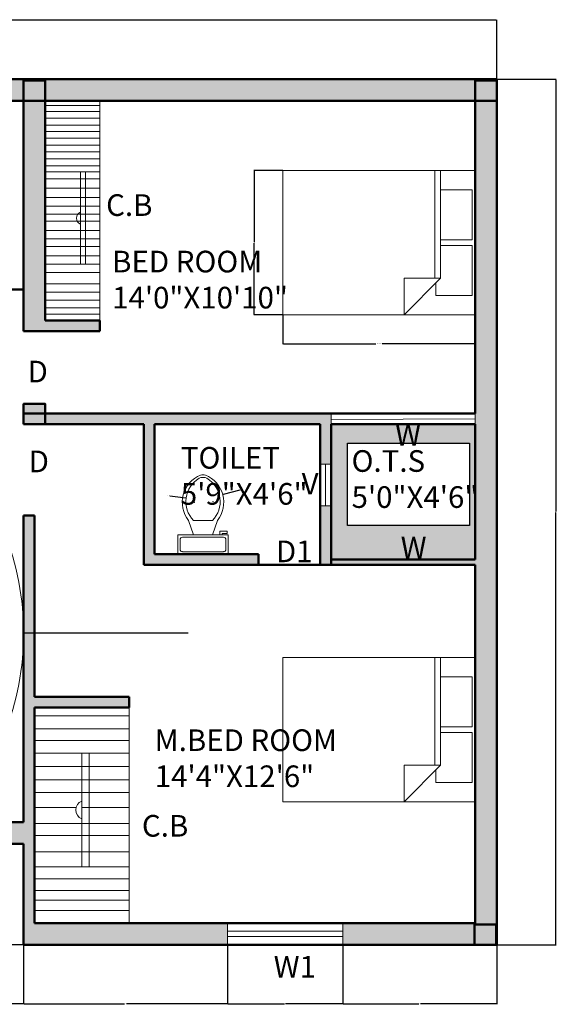
# Model space of a CAD drawing. Units: inches. Extents: x 1099 to 1629, y 1139 to 1548.
# Tile 3 of 3: x 1405 to 1629, y 1139 to 1548. Entities that reach past the tile are written whole.
import ezdxf

# ---------------------------------------------------------------- set-up
doc = ezdxf.new("R2010")
doc.units = ezdxf.units.IN
for name, color, linetype, lineweight in [('A-ANNO-DIMS', 2, 'Continuous', 18), ('A-ANNO-TEXT', 7, 'Continuous', 18), ('A-AREA-IDEN', 7, 'Continuous', 18), ('A-FLOR', 7, 'Continuous', 25), ('A-FLOR-FIXT', 9, 'Continuous', 20), ('A-FLOR-PATT', 3, 'Continuous', 13), ('A-FURN', 8, 'Continuous', 20), ('A-FURN-FIXD', 2, 'Continuous', 18), ('A-WALL', 1, 'Continuous', 50)]:
    doc.layers.add(name, color=color, linetype=linetype, lineweight=lineweight)
for name, color, linetype, lineweight, true_color in [('A-COLS', 177, 'Continuous', 50, 0x293189), ('A-GLAZ', 177, 'Continuous', 20, 0x293189), ('A-WALL-PATT', 244, 'Continuous', 13, 0x991b1e)]:
    doc.layers.add(name, color=color, linetype=linetype, lineweight=lineweight, true_color=true_color)
doc.styles.get("Standard").update_dxf_attribs({"font": 'arial.ttf'})
doc.dimstyles.get("Standard").update_dxf_attribs({"dimtxt": 0.18, "dimasz": 0.18, "dimexe": 0.18, "dimexo": 0.0625, "dimgap": 0.09, "dimtad": 0, "dimtih": 1, "dimtoh": 1, "dimdec": 4, "dimzin": 0, "dimdsep": 46, "dimtxsty": 'Standard', "dimcen": 0.09, "dimadec": 0, "dimazin": 0, "dimtfac": 1, "dimtdec": 4, "dimtofl": 0, "dimtmove": 0, "dimatfit": 3, "dimfxl": 1, "dimtolj": 1, "dimtzin": 0, "dimarcsym": 0})

# ---------------------------------------------------------------- blocks, each defined once
blk = doc.blocks.new('Bed - Queen')
for p, q in [((0, -80.00003), (0, 0)), ((0, 0), (59.99999, 0)), ((59.99999, 0), (59.99999, -80.00003)), ((7.99999, -1.2), (28.79998, -1.2)), ((7.99999, -14.4), (7.99999, -1.2)), ((28.79998, -1.2), (28.79998, -14.4)), ((31.19999, -1.2), (51.99999, -1.2)), ((31.19999, -14.4), (31.19999, -1.2)), ((51.99999, -1.2), (51.99999, -16.4)), ((0, -14.4), (44.8, -14.4)), ((59.99999, -29.6), (44.8, -14.4)), ((44.8, -14.4), (44.8, -29.6)), ((44.8, -16.8), (0, -16.8)), ((51.99999, -16.4), (46.79936, -16.4)), ((44.8, -29.6), (59.99999, -29.6)), ((59.99999, -80.00003), (0, -80.00003))]:
    blk.add_line(p, q)
blk = doc.blocks.new('Toilet - top')
for p, q in [((9.5, -6), (9.5, -2)), ((-8, -8.5), (-8, -8)), ((-7, -8), (-7, -9.5)), ((-4, -8), (-6, -14)), ((4, -8), (6, -14)), ((-10, -8.5), (-8, -8.5)), ((-10, -9.5), (-10, -8.5)), ((-7, -9.5), (-10, -9.5)), ((4, -14), (-4, -14))]:
    blk.add_line(p, q)
blk.add_lwpolyline([(10.5, -8), (10.5, 0), (-10.5, 0), (-10.5, -8)], close=True)
for points in [[(-9.5, -2), (-9.5, -6)], [(8.5, -1), (-8.5, -1)], [(-8.5, -7), (8.5, -7)]]:
    blk.add_lwpolyline(points)
for centre, radius, start, end in [((-8.62, -1.88), 0.884, 81.8699, 188.1301), ((8.62, -1.88), 0.884, 351.8699, 98.1301), ((-8.62, -6.12), 0.884, 171.8699, 278.1301), ((8.62, -6.12), 0.884, 261.8699, 8.1301), ((3.52, -21.58), 12.17, 141.4691, 247.9714), ((4.2, -21.82), 11.33, 136.3677, 238.9468), ((-3.52, -21.58), 12.17, 292.0284, 38.5307), ((-4.2, -21.82), 11.33, 301.053, 43.6321), ((0, -27.88), 4, 245.7318, 294.2682), ((0, -29), 4, 254.8605, 285.1395)]:
    blk.add_arc(centre, radius, start, end)
blk = doc.blocks.new('Sofa - Roundback 7 ft.')
for p, q in [((-12.00002, -32.4421), (-12.00003, -6.5971)), ((11.99997, -32.4421), (11.99998, -6.5971)), ((-36.000027, -34), (-36.000027, -11.4696)), ((35.99998, -34), (35.99998, -11.4696)), ((-35.999844, -13.3819), (35.9998, -13.3819)), ((-36.000027, -32.4421), (35.99998, -32.4421))]:
    blk.add_line(p, q)
for points in [[(-36.000027, -34), (-42.000027, -34), (-42.000027, -8)], [(41.99998, -8), (41.99998, -34), (35.99998, -34)]]:
    blk.add_lwpolyline(points)
for centre, radius, start, end in [((0, -114.25), 114.25, 68.43141, 111.5686), ((-0.00001, -127.1968), 121.1968, 72.72033, 107.2797)]:
    blk.add_arc(centre, radius, start, end)
blk = doc.blocks.new('COL-RECT-9IN')
h = blk.add_hatch(color=256)
h.dxf.hatch_style = 1
h.paths.add_polyline_path([(9, 8.44), (0, 8.44), (0, 0), (9, 0)])
blk.add_lwpolyline([(0, 0), (9, 0), (9, 8.44), (0, 8.44)], close=True)
blk = doc.blocks.new('*D9')
at = {"layer": 'A-ANNO-DIMS', "color": 0, "lineweight": -2, "transparency": 16777216}
for p, q in [((1515.1, 1425.57), (1515.1, 1413.45)), ((1595.1, 1425.57), (1595.1, 1413.45)), ((1515.28, 1413.63), (1553.8, 1413.63)), ((1594.92, 1413.63), (1556.4, 1413.63))]:
    blk.add_line(p, q, dxfattribs=at)
at = {"layer": 'A-ANNO-DIMS', "color": 0, "lineweight": 100, "transparency": 16777216}
for points in [[(1515.28, 1413.66), (1515.28, 1413.6), (1515.1, 1413.63)], [(1594.92, 1413.66), (1594.92, 1413.6), (1595.1, 1413.63)]]:
    blk.add_solid(points, dxfattribs=at)
at = {"layer": 'Defpoints', "color": 0, "lineweight": 100, "transparency": 16777216}
for p in [(1515.1, 1425.63), (1595.1, 1425.63), (1595.1, 1413.63)]:
    blk.add_point(p, dxfattribs=at)
at = {"layer": 'A-ANNO-DIMS', "color": 0, "transparency": 16777216, "insert": (1555.1, 1413.63), "char_height": 0.18, "attachment_point": 5}
blk.add_mtext('\\A1;QUEEN BED 80 TYP.', dxfattribs=at)
blk = doc.blocks.new('*D10')
at = {"layer": 'A-ANNO-DIMS', "color": 0, "lineweight": -2, "transparency": 16777216}
for p, q in [((1515.04, 1485.63), (1502.92, 1485.63)), ((1503.1, 1485.45), (1503.1, 1455.81)), ((1503.1, 1425.81), (1503.1, 1455.45)), ((1515.04, 1425.63), (1502.92, 1425.63))]:
    blk.add_line(p, q, dxfattribs=at)
at = {"layer": 'A-ANNO-DIMS', "color": 0, "lineweight": 100, "transparency": 16777216}
for points in [[(1503.07, 1485.45), (1503.13, 1485.45), (1503.1, 1485.63)], [(1503.07, 1425.81), (1503.13, 1425.81), (1503.1, 1425.63)]]:
    blk.add_solid(points, dxfattribs=at)
at = {"layer": 'Defpoints', "color": 0, "lineweight": 100, "transparency": 16777216}
for p in [(1515.1, 1485.63), (1503.1, 1425.63), (1515.1, 1425.63)]:
    blk.add_point(p, dxfattribs=at)
at = {"layer": 'A-ANNO-DIMS', "color": 0, "transparency": 16777216, "insert": (1503.1, 1455.63), "char_height": 0.18, "attachment_point": 5}
blk.add_mtext('\\A1;60 TYP.', dxfattribs=at)
blk = doc.blocks.new('*D25')
at = {"layer": 'A-ANNO-DIMS', "color": 0, "lineweight": -2, "transparency": 16777216}
for p, q in [((1124.1, 1523.69), (1124.1, 1548.41)), ((1124.28, 1548.23), (1363.81, 1548.23)), ((1603.92, 1548.23), (1364.39, 1548.23)), ((1604.1, 1523.69), (1604.1, 1548.41))]:
    blk.add_line(p, q, dxfattribs=at)
at = {"layer": 'A-ANNO-DIMS', "color": 0, "lineweight": 100, "transparency": 16777216}
for points in [[(1124.28, 1548.26), (1124.28, 1548.2), (1124.1, 1548.23)], [(1603.92, 1548.26), (1603.92, 1548.2), (1604.1, 1548.23)]]:
    blk.add_solid(points, dxfattribs=at)
at = {"layer": 'Defpoints', "color": 0, "lineweight": 100, "transparency": 16777216}
for p in [(1604.1, 1548.23), (1124.1, 1523.63), (1604.1, 1523.63)]:
    blk.add_point(p, dxfattribs=at)
at = {"layer": 'A-ANNO-DIMS', "color": 0, "transparency": 16777216, "insert": (1364.1, 1548.23), "char_height": 0.18, "attachment_point": 5}
blk.add_mtext('\\A1;480', dxfattribs=at)
blk = doc.blocks.new('*D26')
at = {"layer": 'A-ANNO-DIMS', "color": 0, "lineweight": -2, "transparency": 16777216}
for p, q in [((1604.16, 1523.63), (1628.88, 1523.63)), ((1628.7, 1523.45), (1628.7, 1343.81)), ((1628.7, 1163.81), (1628.7, 1343.45)), ((1604.16, 1163.63), (1628.88, 1163.63))]:
    blk.add_line(p, q, dxfattribs=at)
at = {"layer": 'A-ANNO-DIMS', "color": 0, "lineweight": 100, "transparency": 16777216}
for points in [[(1628.67, 1523.45), (1628.73, 1523.45), (1628.7, 1523.63)], [(1628.67, 1163.81), (1628.73, 1163.81), (1628.7, 1163.63)]]:
    blk.add_solid(points, dxfattribs=at)
at = {"layer": 'Defpoints', "color": 0, "lineweight": 100, "transparency": 16777216}
for p in [(1604.1, 1523.63), (1628.7, 1523.63), (1604.1, 1163.63)]:
    blk.add_point(p, dxfattribs=at)
at = {"layer": 'A-ANNO-DIMS', "color": 0, "transparency": 16777216, "insert": (1628.7, 1343.63), "char_height": 0.18, "attachment_point": 5}
blk.add_mtext('\\A1;360', dxfattribs=at)
blk = doc.blocks.new('*D30')
at = {"layer": 'A-ANNO-DIMS', "color": 0, "lineweight": -2, "transparency": 16777216}
for p, q in [((1386.73, 1205.57), (1386.73, 1138.85)), ((1407.1, 1163.57), (1407.1, 1138.85)), ((1386.91, 1139.03), (1396.52, 1139.03)), ((1406.92, 1139.03), (1397.31, 1139.03))]:
    blk.add_line(p, q, dxfattribs=at)
at = {"layer": 'A-ANNO-DIMS', "color": 0, "lineweight": 100, "transparency": 16777216}
for points in [[(1386.91, 1139.06), (1386.91, 1139), (1386.73, 1139.03)], [(1406.92, 1139.06), (1406.92, 1139), (1407.1, 1139.03)]]:
    blk.add_solid(points, dxfattribs=at)
at = {"layer": 'Defpoints', "color": 0, "lineweight": 100, "transparency": 16777216}
for p in [(1386.73, 1205.63), (1407.1, 1163.63), (1407.1, 1139.03)]:
    blk.add_point(p, dxfattribs=at)
at = {"layer": 'A-ANNO-DIMS', "color": 0, "transparency": 16777216, "insert": (1396.91, 1139.03), "char_height": 0.18, "attachment_point": 5}
blk.add_mtext('\\A1;20.37', dxfattribs=at)
blk = doc.blocks.new('*D31')
at = {"layer": 'A-ANNO-DIMS', "color": 0, "lineweight": -2, "transparency": 16777216}
for p, q in [((1407.1, 1163.57), (1407.1, 1138.85)), ((1491.99, 1163.57), (1491.99, 1138.85)), ((1407.28, 1139.03), (1449.15, 1139.03)), ((1491.81, 1139.03), (1449.94, 1139.03))]:
    blk.add_line(p, q, dxfattribs=at)
at = {"layer": 'A-ANNO-DIMS', "color": 0, "lineweight": 100, "transparency": 16777216}
for points in [[(1407.28, 1139.06), (1407.28, 1139), (1407.1, 1139.03)], [(1491.81, 1139.06), (1491.81, 1139), (1491.99, 1139.03)]]:
    blk.add_solid(points, dxfattribs=at)
at = {"layer": 'Defpoints', "color": 0, "lineweight": 100, "transparency": 16777216}
for p in [(1407.1, 1163.63), (1491.99, 1163.63), (1491.99, 1139.03)]:
    blk.add_point(p, dxfattribs=at)
at = {"layer": 'A-ANNO-DIMS', "color": 0, "transparency": 16777216, "insert": (1449.54, 1139.03), "char_height": 0.18, "attachment_point": 5}
blk.add_mtext('\\A1;84.89', dxfattribs=at)
blk = doc.blocks.new('*D32')
at = {"layer": 'A-ANNO-DIMS', "color": 0, "lineweight": -2, "transparency": 16777216}
for p, q in [((1491.99, 1163.57), (1491.99, 1138.85)), ((1539.99, 1163.57), (1539.99, 1138.85)), ((1492.17, 1139.03), (1515.77, 1139.03)), ((1539.81, 1139.03), (1516.21, 1139.03))]:
    blk.add_line(p, q, dxfattribs=at)
at = {"layer": 'A-ANNO-DIMS', "color": 0, "lineweight": 100, "transparency": 16777216}
for points in [[(1492.17, 1139.06), (1492.17, 1139), (1491.99, 1139.03)], [(1539.81, 1139.06), (1539.81, 1139), (1539.99, 1139.03)]]:
    blk.add_solid(points, dxfattribs=at)
at = {"layer": 'Defpoints', "color": 0, "lineweight": 100, "transparency": 16777216}
for p in [(1491.99, 1163.63), (1539.99, 1163.63), (1539.99, 1139.03)]:
    blk.add_point(p, dxfattribs=at)
at = {"layer": 'A-ANNO-DIMS', "color": 0, "transparency": 16777216, "insert": (1515.99, 1139.03), "char_height": 0.18, "attachment_point": 5}
blk.add_mtext('\\A1;48', dxfattribs=at)
blk = doc.blocks.new('*D33')
at = {"layer": 'A-ANNO-DIMS', "color": 0, "lineweight": -2, "transparency": 16777216}
for p, q in [((1539.99, 1163.57), (1539.99, 1138.85)), ((1604.1, 1163.57), (1604.1, 1138.85)), ((1540.17, 1139.03), (1571.67, 1139.03)), ((1603.92, 1139.03), (1572.42, 1139.03))]:
    blk.add_line(p, q, dxfattribs=at)
at = {"layer": 'A-ANNO-DIMS', "color": 0, "lineweight": 100, "transparency": 16777216}
for points in [[(1540.17, 1139.06), (1540.17, 1139), (1539.99, 1139.03)], [(1603.92, 1139.06), (1603.92, 1139), (1604.1, 1139.03)]]:
    blk.add_solid(points, dxfattribs=at)
at = {"layer": 'Defpoints', "color": 0, "lineweight": 100, "transparency": 16777216}
for p in [(1539.99, 1163.63), (1604.1, 1163.63), (1604.1, 1139.03)]:
    blk.add_point(p, dxfattribs=at)
at = {"layer": 'A-ANNO-DIMS', "color": 0, "transparency": 16777216, "insert": (1572.04, 1139.03), "char_height": 0.18, "attachment_point": 5}
blk.add_mtext('\\A1;64.11', dxfattribs=at)
blk = doc.blocks.new('*D38')
at = {"layer": 'A-ANNO-DIMS', "color": 0, "lineweight": -2, "transparency": 16777216}
for p, q in [((1292.76, 1293.22), (1292.94, 1293.22)), ((1292.85, 1293.13), (1292.85, 1293.31)), ((1475.65, 1293.22), (1407.28, 1293.22))]:
    blk.add_line(p, q, dxfattribs=at)
at = {"layer": 'A-ANNO-DIMS', "color": 0, "lineweight": 100, "transparency": 16777216}
blk.add_solid([(1407.28, 1293.25), (1407.28, 1293.19), (1407.1, 1293.22)], dxfattribs=at)
at = {"layer": 'Defpoints', "color": 0, "lineweight": 100, "transparency": 16777216}
for p in [(1292.85, 1293.22), (1407.1, 1293.22)]:
    blk.add_point(p, dxfattribs=at)
at = {"layer": 'A-ANNO-DIMS', "color": 0, "transparency": 16777216, "insert": (1476.39, 1293.22), "char_height": 0.18, "attachment_point": 5}
blk.add_mtext('\\A1;2X R114.25', dxfattribs=at)
blk = doc.blocks.new('*D40')
at = {"layer": 'A-ANNO-DIMS', "color": 0, "lineweight": -2, "transparency": 16777216}
for p, q in [((1497.11, 1352.66), (1490.22, 1350.85)), ((1478.19, 1347.71), (1478.37, 1347.71)), ((1478.28, 1347.62), (1478.28, 1347.8))]:
    blk.add_line(p, q, dxfattribs=at)
at = {"layer": 'A-ANNO-DIMS', "color": 0, "lineweight": 100, "transparency": 16777216}
blk.add_solid([(1490.21, 1350.88), (1490.23, 1350.82), (1490.05, 1350.8)], dxfattribs=at)
at = {"layer": 'Defpoints', "color": 0, "lineweight": 100, "transparency": 16777216}
for p in [(1478.28, 1347.71), (1490.05, 1350.8)]:
    blk.add_point(p, dxfattribs=at)
at = {"layer": 'A-ANNO-DIMS', "color": 0, "transparency": 16777216, "insert": (1497.78, 1352.66), "char_height": 0.18, "attachment_point": 5}
blk.add_mtext('\\A1;4X R12.17', dxfattribs=at)
blk = doc.blocks.new('*D41')
at = {"layer": 'A-ANNO-DIMS', "color": 0, "lineweight": -2, "transparency": 16777216}
for p, q in [((1468.03, 1350.36), (1474.59, 1349.48)), ((1485.9, 1347.95), (1486.08, 1347.95)), ((1485.99, 1347.86), (1485.99, 1348.04))]:
    blk.add_line(p, q, dxfattribs=at)
at = {"layer": 'A-ANNO-DIMS', "color": 0, "lineweight": 100, "transparency": 16777216}
blk.add_solid([(1474.59, 1349.51), (1474.58, 1349.45), (1474.77, 1349.46)], dxfattribs=at)
at = {"layer": 'Defpoints', "color": 0, "lineweight": 100, "transparency": 16777216}
for p in [(1474.77, 1349.46), (1485.99, 1347.95)]:
    blk.add_point(p, dxfattribs=at)
at = {"layer": 'A-ANNO-DIMS', "color": 0, "transparency": 16777216, "insert": (1467.35, 1350.36), "char_height": 0.18, "attachment_point": 5}
blk.add_mtext('\\A1;4X R11.33', dxfattribs=at)

msp = doc.modelspace()

# ---------------------------------------------------------------- hatches: boundary and pattern name
at = {"layer": 'A-FLOR-PATT'}
h = msp.add_hatch(color=256, dxfattribs=at)
h.dxf.hatch_style = 1
h.paths.add_polyline_path([(1595.099, 1380.128), (1535.099, 1380.128), (1535.099, 1326.128), (1535.099, 1323.878), (1595.099, 1323.878)])
h.paths.add_polyline_path([(1542.026, 1338.035), (1542.026, 1372.311), (1592.789, 1372.311), (1592.789, 1338.035)], flags=16)
h.paths.add_polyline_path([(1540.803, 1340.228), (1595.472, 1340.228), (1595.472, 1373.811), (1540.803, 1373.811)], flags=9)
at = {"layer": 'A-WALL-PATT'}
h = msp.add_hatch(color=256, dxfattribs=at)
h.dxf.hatch_style = 1
h.paths.add_polyline_path([(1407.099, 1523.072), (1416.099, 1523.072), (1416.099, 1514.628), (1595.099, 1514.628), (1595.099, 1523.072), (1604.099, 1523.072), (1604.099, 1523.628), (1124.099, 1523.628), (1124.099, 1172.072), (1133.099, 1172.072), (1133.099, 1361.628), (1265.099, 1361.628), (1265.099, 1301.628), (1269.599, 1301.628), (1269.599, 1366.128), (1133.099, 1366.128), (1133.099, 1462.128), (1169.127, 1462.128), (1169.127, 1466.628), (1133.099, 1466.628), (1133.099, 1514.628), (1265.099, 1514.628), (1265.099, 1514.872), (1265.099, 1523.316), (1274.099, 1523.316), (1274.099, 1514.628), (1326.599, 1514.628), (1326.599, 1508.465), (1331.099, 1508.465), (1331.099, 1514.628), (1407.099, 1514.628)])
h.paths.add_polyline_path([(1604.099, 1514.628), (1595.099, 1514.628), (1595.099, 1384.628), (1595.099, 1380.128), (1595.099, 1323.878), (1535.099, 1323.878), (1535.099, 1321.628), (1595.099, 1321.628), (1595.099, 1172.628), (1539.988, 1172.628), (1539.988, 1163.628), (1594.904, 1163.628), (1594.904, 1172.072), (1604.099, 1172.072)])
h.paths.add_polyline_path([(1461.599, 1380.128), (1530.599, 1380.128), (1530.599, 1363.564), (1535.099, 1363.564), (1535.099, 1380.128), (1535.099, 1384.628), (1416.099, 1384.628), (1416.099, 1380.128), (1457.099, 1380.128), (1457.099, 1326.128), (1457.099, 1321.628), (1504.951, 1321.628), (1504.951, 1326.128), (1461.599, 1326.128)], flags=17)
h.paths.add_polyline_path([(1535.099, 1346.252), (1530.599, 1346.252), (1530.599, 1326.128), (1530.599, 1321.628), (1535.099, 1321.628), (1535.099, 1323.878), (1535.099, 1326.128)], flags=16)
h.paths.add_polyline_path([(1269.599, 1301.628), (1265.099, 1301.628), (1260.599, 1301.628), (1260.599, 1214.628), (1260.599, 1205.628), (1265.099, 1205.628), (1269.599, 1205.628), (1269.599, 1214.628)], flags=17)
h.paths.add_polyline_path([(1411.599, 1262.279), (1451.001, 1262.279), (1451.001, 1266.779), (1411.599, 1266.779), (1411.599, 1342.184), (1407.099, 1342.184), (1407.099, 1214.628), (1386.727, 1214.628), (1386.727, 1205.628), (1407.099, 1205.628), (1407.099, 1163.628), (1491.988, 1163.628), (1491.988, 1172.628), (1411.599, 1172.628)])
h.paths.add_polyline_path([(1315.906, 1214.628), (1300.958, 1214.628), (1300.958, 1205.628), (1315.906, 1205.628)], flags=17)
h = msp.add_hatch(color=256, dxfattribs=at)
h.dxf.hatch_style = 1
h.paths.add_polyline_path([(1233.806, 1466.628), (1205.127, 1466.628), (1205.127, 1462.128), (1233.806, 1462.128)])
h.paths.add_polyline_path([(1269.599, 1486.628), (1289.77, 1486.628), (1289.77, 1491.128), (1269.599, 1491.128), (1265.099, 1491.128), (1265.099, 1400.307), (1269.599, 1400.307)])
h.paths.add_polyline_path([(1379.104, 1440.628), (1331.099, 1440.628), (1331.099, 1498.77), (1326.599, 1498.77), (1326.599, 1491.128), (1310.198, 1491.128), (1310.198, 1486.628), (1326.599, 1486.628), (1326.599, 1440.628), (1291.317, 1440.628), (1291.317, 1436.128), (1379.104, 1436.128)])
h.paths.add_polyline_path([(1416.099, 1514.628), (1407.099, 1514.628), (1407.099, 1418.838), (1411.599, 1418.838), (1438.846, 1418.838), (1438.846, 1423.338), (1416.099, 1423.338)])

# ---------------------------------------------------------------- linework, layer by layer
at = {"layer": 'A-FLOR'}
msp.add_line((1407.099, 1163.628), (1133.099, 1163.628), dxfattribs=at)
msp.add_lwpolyline([(1542.026, 1372.311), (1592.789, 1372.311), (1592.789, 1338.035), (1542.026, 1338.035)], close=True, dxfattribs=at)
at = {"layer": 'A-FURN-FIXD'}
for p, q in [((1438.846, 1512.736), (1416.099, 1512.736)), ((1438.846, 1423.338), (1438.846, 1514.628)), ((1438.846, 1510.279), (1416.099, 1510.279)), ((1438.846, 1507.44), (1416.099, 1507.44)), ((1438.846, 1504.6), (1416.099, 1504.6)), ((1438.846, 1501.962), (1416.099, 1501.962)), ((1438.846, 1499.176), (1416.099, 1499.176)), ((1438.846, 1496.28), (1416.099, 1496.28)), ((1438.846, 1493.478), (1416.099, 1493.478)), ((1438.846, 1490.473), (1416.099, 1490.473)), ((1438.846, 1487.633), (1416.099, 1487.633)), ((1438.846, 1485.065), (1416.099, 1485.065)), ((1438.846, 1482.279), (1416.099, 1482.279)), ((1438.846, 1478.294), (1416.099, 1478.294)), ((1438.846, 1474.492), (1416.099, 1474.492)), ((1438.846, 1470.825), (1416.099, 1470.825)), ((1438.846, 1467.501), (1416.099, 1467.501)), ((1438.846, 1464.615), (1416.099, 1464.615)), ((1438.846, 1460.771), (1416.099, 1460.771)), ((1438.846, 1457.189), (1416.099, 1457.189)), ((1438.846, 1454.054), (1416.099, 1454.054)), ((1438.846, 1450.248), (1416.099, 1450.248)), ((1438.846, 1446.666), (1416.099, 1446.666)), ((1438.846, 1443.307), (1416.099, 1443.307)), ((1438.846, 1438.605), (1416.099, 1438.605)), ((1438.846, 1435.018), (1416.099, 1435.018)), ((1438.846, 1431.689), (1416.099, 1431.689)), ((1438.846, 1428.536), (1416.099, 1428.536)), ((1438.846, 1425.908), (1416.099, 1425.908)), ((1451.001, 1262.279), (1451.001, 1172.628)), ((1411.599, 1258.872), (1451.001, 1258.872)), ((1411.599, 1253.396), (1451.001, 1253.396)), ((1411.599, 1248.52), (1451.001, 1248.52)), ((1411.599, 1243.365), (1451.001, 1243.365)), ((1411.599, 1237.792), (1451.001, 1237.792)), ((1411.599, 1232.219), (1451.001, 1232.219)), ((1411.599, 1226.899), (1451.001, 1226.899)), ((1411.599, 1220.769), (1428.994, 1220.769)), ((1434.381, 1220.769), (1431.3, 1220.769)), ((1434.381, 1220.769), (1451.001, 1220.769)), ((1411.599, 1214.082), (1451.001, 1214.082)), ((1411.599, 1209.066), (1451.001, 1209.066)), ((1411.599, 1202.226), (1451.001, 1202.226)), ((1411.599, 1195.985), (1451.001, 1195.985)), ((1411.599, 1191.082), (1451.001, 1191.082)), ((1411.599, 1186.178), (1451.001, 1186.178)), ((1411.599, 1182.166), (1451.001, 1182.166)), ((1411.599, 1177.931), (1451.001, 1177.931))]:
    msp.add_line(p, q, dxfattribs=at)
for points in [[(1432.896, 1485.065), (1430.79, 1485.065), (1430.79, 1446.666), (1432.896, 1446.666)], [(1431.3, 1243.365), (1434.381, 1243.365), (1434.381, 1195.985), (1431.3, 1195.985)]]:
    msp.add_lwpolyline(points, close=True, dxfattribs=at)
for centre, radius, start, end in [((1431.843, 1465.865), 2.684, 113.09565, 246.90435), ((1432.84, 1219.675), 3.999, 112.66152, 247.33848)]:
    msp.add_arc(centre, radius, start, end, dxfattribs=at)
at = {"layer": 'A-GLAZ'}
for p, q in [((1535.099, 1380.128), (1535.099, 1384.628)), ((1595.099, 1380.128), (1595.099, 1384.628)), ((1595.099, 1382.378), (1535.099, 1382.066)), ((1535.099, 1363.564), (1530.599, 1363.564)), ((1532.849, 1346.252), (1532.849, 1363.564)), ((1535.099, 1346.252), (1530.599, 1346.252)), ((1491.988, 1172.628), (1491.988, 1163.628)), ((1539.988, 1172.628), (1539.988, 1163.628)), ((1491.988, 1169.335), (1539.988, 1169.335)), ((1491.988, 1167.058), (1539.988, 1167.058))]:
    msp.add_line(p, q, dxfattribs=at)
at = {"layer": 'A-WALL'}
for p, q in [((1604.099, 1523.628), (1124.099, 1523.628)), ((1604.099, 1163.628), (1604.099, 1523.628)), ((1407.099, 1514.628), (1331.099, 1514.628)), ((1407.099, 1514.628), (1407.099, 1418.838)), ((1595.099, 1514.628), (1416.099, 1514.628)), ((1416.099, 1514.628), (1416.099, 1423.338)), ((1595.099, 1384.628), (1595.099, 1514.628)), ((1407.099, 1440.628), (1407.099, 1436.128)), ((1407.099, 1436.128), (1269.599, 1436.128)), ((1438.846, 1423.338), (1416.099, 1423.338)), ((1438.846, 1418.838), (1438.846, 1423.338)), ((1411.599, 1418.838), (1407.099, 1418.838)), ((1411.599, 1418.838), (1438.846, 1418.838)), ((1595.099, 1384.628), (1407.099, 1384.628)), ((1407.099, 1384.628), (1407.099, 1380.128)), ((1407.099, 1384.628), (1407.099, 1380.128)), ((1457.099, 1380.128), (1407.099, 1380.128)), ((1457.099, 1326.128), (1457.099, 1380.128)), ((1461.599, 1326.128), (1461.599, 1380.128)), ((1530.599, 1380.128), (1461.599, 1380.128)), ((1530.599, 1326.128), (1530.599, 1380.128)), ((1595.099, 1380.128), (1535.099, 1380.128)), ((1535.099, 1326.128), (1535.099, 1380.128)), ((1595.099, 1323.878), (1595.099, 1380.128)), ((1411.599, 1342.184), (1407.099, 1342.184)), ((1407.099, 1342.184), (1407.099, 1214.628)), ((1411.599, 1342.184), (1411.599, 1266.779)), ((1457.099, 1326.128), (1457.099, 1321.628)), ((1504.951, 1326.128), (1461.599, 1326.128)), ((1504.951, 1326.128), (1504.951, 1321.628)), ((1530.599, 1326.128), (1530.599, 1321.628)), ((1535.099, 1326.128), (1535.099, 1321.628)), ((1535.099, 1323.878), (1595.099, 1323.878)), ((1595.099, 1321.628), (1457.099, 1321.628)), ((1595.099, 1172.628), (1595.099, 1321.628)), ((1411.599, 1266.779), (1451.001, 1266.779)), ((1451.001, 1266.779), (1451.001, 1262.279)), ((1451.001, 1262.279), (1411.599, 1262.279)), ((1411.599, 1262.279), (1411.599, 1172.628)), ((1300.958, 1214.628), (1407.099, 1214.628)), ((1265.099, 1205.628), (1407.099, 1205.628)), ((1407.099, 1205.628), (1407.099, 1163.628)), ((1411.599, 1172.628), (1595.099, 1172.628)), ((1407.099, 1163.628), (1604.099, 1163.628))]:
    msp.add_line(p, q, dxfattribs=at)

# ---------------------------------------------------------------- block references
at = {"layer": 'A-COLS'}
for p in [(1407.099, 1514.628), (1595.099, 1514.628), (1407.099, 1380.128), (1594.904, 1163.628)]:
    msp.add_blockref('COL-RECT-9IN', p, dxfattribs=at)
at = {"layer": 'A-FLOR-FIXT', "rotation": 180}
msp.add_blockref('Toilet - top', (1481.795, 1326.128), dxfattribs=at)
at = {"layer": 'A-FURN', "rotation": 270}
for name, p in [('Bed - Queen', (1595.099, 1485.629)), ('Sofa - Roundback 7 ft.', (1407.099, 1293.22)), ('Bed - Queen', (1595.099, 1283.126))]:
    msp.add_blockref(name, p, dxfattribs=at)

# ---------------------------------------------------------------- texts
at = {"layer": 'A-ANNO-TEXT', "char_height": 9, "attachment_point": 1}
for s, insert in [('C.B', (1441.452, 1475.785)), ('D', (1408.74, 1406.542)), ('W', (1561.774, 1380.269)), ('D', (1409.198, 1369.161)), ('V', (1522.864, 1359.916)), ('D1', (1512.134, 1331.748)), ('W', (1564.102, 1333.341)), ('C.B', (1456.374, 1217.595)), ('W1', (1511.224, 1158.98))]:
    msp.add_mtext_dynamic_manual_height_columns(s, width=16.11456, gutter_width=12.5, heights=[0], dxfattribs=dict(at, insert=insert))
at = {"layer": 'A-AREA-IDEN', "char_height": 9, "attachment_point": 1}
for s, width, insert in [('BED ROOM\\P14\'0"X10\'10"', 95.09467, (1443.952, 1452.295)), ('TOILET\\P5\'9"X4\'6"', 79.89808, (1472.565, 1370.663)), ('O.T.S\\P5\'0"X4\'6"', 79.89808, (1543.661, 1369.338)), ('M.BED ROOM\\P14\'4"X12\'6"', 91.32581, (1461.695, 1253.203))]:
    msp.add_mtext_dynamic_manual_height_columns(s, width=width, gutter_width=12.5, heights=[0], dxfattribs=dict(at, insert=insert))

# ---------------------------------------------------------------- dimensions: what is measured, and where the dimension line sits
at = {"layer": 'A-ANNO-DIMS'}
for base, p1, p2, override, picture, middle in [((1604.099, 1548.228), (1124.099, 1523.628), (1604.099, 1523.628), {"dimdec": 0, "dimlfac": 1, "dimrnd": 0, "dimzin": 0, "dimdsep": 46, "dimlunit": 2}, '*D25', (1364.099, 1548.228)), ((1407.099, 1139.028), (1386.727, 1205.628), (1407.099, 1163.628), {"dimdec": 2, "dimlfac": 1, "dimrnd": 0, "dimzin": 0, "dimdsep": 46, "dimlunit": 2}, '*D30', (1396.913, 1139.028)), ((1491.988, 1139.028), (1407.099, 1163.628), (1491.988, 1163.628), {"dimdec": 2, "dimlfac": 1, "dimrnd": 0, "dimzin": 0, "dimdsep": 46, "dimlunit": 2}, '*D31', (1449.544, 1139.028)), ((1539.988, 1139.028), (1491.988, 1163.628), (1539.988, 1163.628), {"dimdec": 0, "dimlfac": 1, "dimrnd": 0, "dimzin": 0, "dimdsep": 46, "dimlunit": 2}, '*D32', (1515.988, 1139.028)), ((1604.099, 1139.028), (1539.988, 1163.628), (1604.099, 1163.628), {"dimdec": 2, "dimlfac": 1, "dimrnd": 0, "dimzin": 0, "dimdsep": 46, "dimlunit": 2}, '*D33', (1572.044, 1139.028))]:
    dim = msp.add_linear_dim(base=base, p1=p1, p2=p2, dimstyle='Standard', override=override, dxfattribs=at)
    dim.commit()
    dim.dimension.update_dxf_attribs({"geometry": picture, "text_midpoint": middle})
dim = msp.add_linear_dim(base=(1628.699, 1523.628), p1=(1604.099, 1163.628), p2=(1604.099, 1523.628), angle=90, dimstyle='Standard', override={"dimdec": 0, "dimlfac": 1, "dimrnd": 0, "dimzin": 0, "dimdsep": 46, "dimlunit": 2}, dxfattribs=at)
dim.commit()
dim.dimension.update_dxf_attribs({"geometry": '*D26', "text_midpoint": (1628.699, 1343.628)})
dim = msp.add_linear_dim(base=(1503.099, 1425.629), p1=(1515.099, 1485.629), p2=(1515.099, 1425.629), angle=270, text='<> TYP.', dimstyle='Standard', override={"dimdec": 0, "dimlfac": 1, "dimrnd": 0, "dimzin": 0, "dimdsep": 46, "dimlunit": 2}, dxfattribs=at)
dim.commit()
dim.dimension.update_dxf_attribs({"geometry": '*D10', "text_midpoint": (1503.099, 1455.629)})
dim = msp.add_linear_dim(base=(1595.099, 1413.629), p1=(1515.099, 1425.629), p2=(1595.099, 1425.629), text='QUEEN BED <> TYP.', dimstyle='Standard', override={"dimdec": 0, "dimlfac": 1, "dimrnd": 0, "dimzin": 0, "dimdsep": 46, "dimlunit": 2}, dxfattribs=at)
dim.commit()
dim.dimension.update_dxf_attribs({"geometry": '*D9', "text_midpoint": (1555.099, 1413.629)})
for center, mpoint, text, picture, middle in [((1478.275, 1347.708), (1490.045, 1350.801), '4X <>', '*D40', (1497.107, 1352.657)), ((1485.995, 1347.945), (1474.767, 1349.455), '4X <>', '*D41', (1468.03, 1350.361)), ((1292.849, 1293.22), (1407.099, 1293.22), '2X <>', '*D38', (1475.649, 1293.22))]:
    dim = msp.add_radius_dim(center=center, mpoint=mpoint, text=text, dimstyle='Standard', override={"dimdec": 2, "dimlfac": 1, "dimrnd": 0, "dimzin": 0, "dimdsep": 46, "dimlunit": 2}, dxfattribs=at)
    dim.commit()
    dim.dimension.update_dxf_attribs({"geometry": picture, "text_midpoint": middle, "dimtype": 164})

doc.saveas('drawing.dxf')
